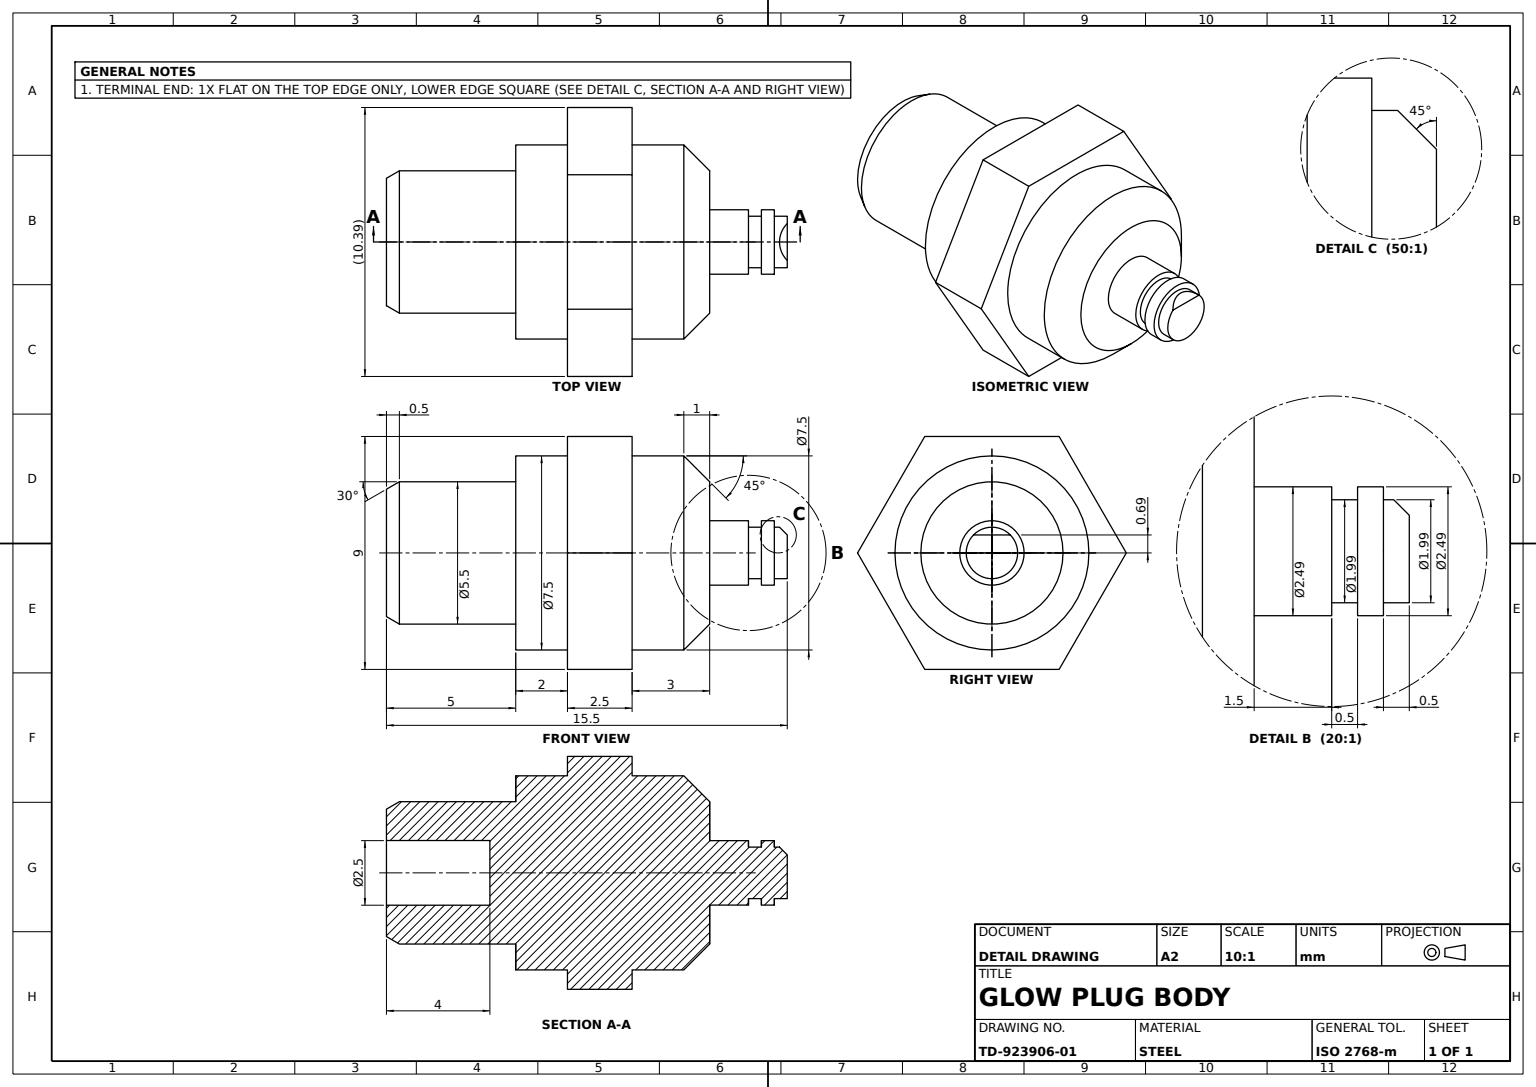
SolidWorks part; units mm, degrees
material "Plain Carbon Steel"
ref_plane "Front Plane" through (0, 0, 0) normal (0, 0, 1) x (1, 0, 0)
ref_plane "Top Plane" through (0, 0, 0) normal (0, 1, 0) x (1, 0, 0)
ref_plane "Right Plane" through (0, 0, 0) normal (1, 0, 0) x (0, 0, -1)
sketch "Hex Profile 9AF Sketch" plane through (0, 0, 0) normal (0, 0, 1) x (1, 0, 0)
  line L1 (2.5981, 4.5) -> (-2.5981, 4.5)
  line L2 (-2.5981, 4.5) -> (-5.1962, 0)
  line L3 (-5.1962, 0) -> (-2.5981, -4.5)
  line L4 (-2.5981, -4.5) -> (2.5981, -4.5)
  line L5 (2.5981, -4.5) -> (5.1962, 0)
  line L6 (5.1962, 0) -> (2.5981, 4.5)
  circle A0 centre (0, 0) radius 4.5 construction
  dimension "D1" = 9
extrude "Hex Body 9AF" add sketch "Hex Profile 9AF Sketch" along normal blind 2.5
sketch "Collar Ø7.5 Sketch" plane through (0, 0, 2.5) normal (0, 0, 1) x (1, 0, 0)
  circle A0 centre (0, 0) radius 3.75
  dimension "D1" = 7.5
extrude "Collar Ø7.5" add sketch "Collar Ø7.5 Sketch" along normal blind 2 contours A0
sketch "Tip Body Ø5.5 Sketch" plane through (0, 0, 4.5) normal (0, 0, 1) x (1, 0, 0)
  circle A0 centre (0, 0) radius 2.75
  dimension "D1" = 5.5
extrude "Tip Body Ø5.5" add sketch "Tip Body Ø5.5 Sketch" along normal blind 5
chamfer "Tip End Chamfer 0.5x30" distance 0.5 angle 30 1 edges at (2.75, 0, 9.5)
sketch "Tip Bore Ø2.5 Sketch" plane through (0, 0, 9.5) normal (0, 0, 1) x (1, 0, 0)
  circle A0 centre (0, 0) radius 1.25
  dimension "D1" = 2.5
extrude "Tip Bore Ø2.5" cut sketch "Tip Bore Ø2.5 Sketch" against normal blind 4
sketch "Shank Ø7.5 Sketch" plane through (0, 0, 0) normal (0, 0, -1) x (-1, 0, 0)
  circle A0 centre (0, 0) radius 3.75
  dimension "D1" = 7.5
extrude "Shank Ø7.5" add sketch "Shank Ø7.5 Sketch" along normal blind 3
chamfer "Shank Chamfer 1x45" distance 1 angle 45 1 edges at (-3.75, 0, -3)
sketch "Terminal Stud Profile Sketch" plane through (0, 0, 0) normal (1, 0, 0) x (0, 0, -1)
  line L0 (3, -2.75) -> (3, 2.75) construction
  line L1 (3, -2.75) -> (3, 2.75) construction
  line L2 (3, 0) -> (6, 0) construction
  line L3 (3, -1.245) -> (4.5, -1.245)
  line L4 (4.5, -1.245) -> (4.5, -0.995)
  line L5 (4.5, -0.995) -> (5, -0.995)
  line L6 (5, -0.995) -> (5, -1.245)
  line L7 (5, -1.245) -> (5.5, -1.245)
  line L8 (5.5, -1.245) -> (5.5, -0.995)
  line L9 (5.5, -0.995) -> (6, -0.995)
  line L10 (6, -0.995) -> (6, 0)
  line L11 (3, 0) -> (6, 0)
  line L12 (3, 0) -> (3, -1.245)
  dimension "D1" = 1.245
  dimension "D2" = 0.25
  dimension "D3" = 0.5
  dimension "D4" = 0.25
  dimension "D5" = 0.5
  dimension "D6" = 0.25
  dimension "D7" = 1.5
  dimension "D8" = 3
revolve "Terminal Stud" add sketch "Terminal Stud Profile Sketch" angle 360 about L11
sketch "Terminal Notch Sketch" plane through (0, 0, 0) normal (1, 0, 0) x (0, 0, -1)
  line L0 (6, 0.695) -> (5.7, 0.995)
  line L1 (6, -0.995) -> (6, 0.995) construction
  line L2 (6, 0.695) -> (6, 0.995)
  line L3 (6, 0.995) -> (5.5, 0.995) construction
  line L4 (6, 0.995) -> (5.7, 0.995)
  dimension "D2" = 0.3
  dimension "D3" = 0.4243
extrude "Terminal Notch Cut" cut sketch "Terminal Notch Sketch" against normal through all both and the other way through all
